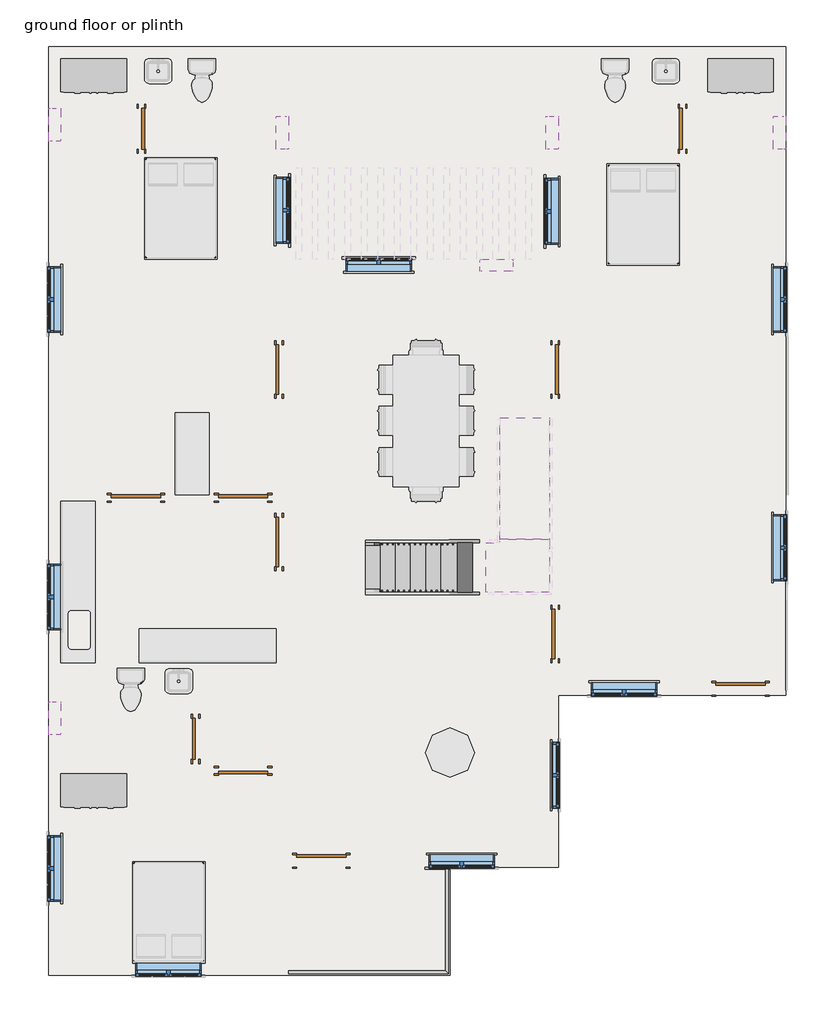
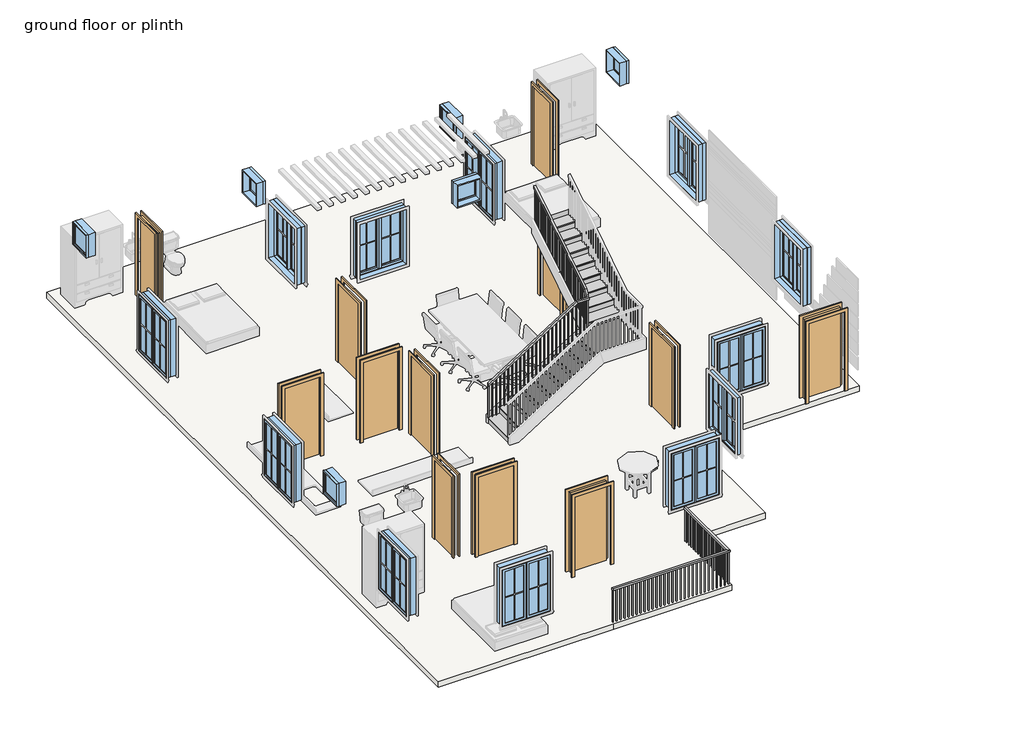
# One storey, part 1 of 3: 18 windows, 12 doors, 2 railings, 2 slabs, 2 stair flights.
"""IFC4 building model written with IfcOpenShell, lengths in millimetres."""

from ifc_helpers import new_model, si_unit, frame, origin, place, context, project, spatial, polyline, outline, extrude, faceted_brep, transform, mapped, element, save
from components import door_78caadf7, door_214872d5, door_e5f9f3c4, door_305aa2a5, door_0ca8825f, door_a90ba1ad, non_monolithic_landing_c5e4f846, stair_flight_fd6a9547, stair_flight_b3cbfaaf, window_80340324, window_8377141f, window_d9d3dda5

model = new_model("IFC4")

# Units and contexts
model_context = context("Model", 3, world=origin())
ifc_project = project(units=[si_unit("LENGTHUNIT", "METRE", prefix="MILLI")], contexts=[model_context])

# Site, building, storey
site = spatial("IfcSite", under=ifc_project)
building = spatial("IfcBuilding", under=site)
storey = spatial("IfcBuildingStorey", under=building, Name="ground floor or plinth", Elevation=609.6)

# Doors
placement = place(None, origin())
door_shape = door_78caadf7(model_context)
element("IfcDoor", 1, ObjectType="Single-Flush : 30\" x 84\"", at=placement, inside=storey, context=model_context, shape_type="MappedRepresentation", body=[
    mapped(door_shape, transform((3433.3423267, 4208.8496924, 609.6), x_axis=(0.0, -1.0, 0.0), y_axis=(1.0, 0.0, 0.0), z_axis=(0.0, 0.0, 1.0))),
])
element("IfcDoor", 2, ObjectType="Single-Flush : 30\" x 84\"", at=placement, inside=storey, context=model_context, shape_type="MappedRepresentation", body=[
    mapped(door_shape, transform((12463.0423267, 15511.8496924, 609.6), x_axis=(0.0, -1.0, 0.0), y_axis=(1.0, 0.0, 0.0), z_axis=(0.0, 0.0, 1.0))),
])
door_2_shape = door_214872d5(model_context)
element("IfcDoor", 3, ObjectType="Single-Flush : 30\" x 84\"", at=placement, inside=storey, context=model_context, shape_type="MappedRepresentation", body=[
    mapped(door_2_shape, transform((2430.0423267, 15511.8496924, 609.6), x_axis=(0.0, -1.0, 0.0), y_axis=(1.0, 0.0, 0.0), z_axis=(0.0, 0.0, 1.0))),
])
door_3_shape = door_e5f9f3c4(model_context)
element("IfcDoor", 4, ObjectType="Single-Flush : 36\" x 84\"", at=placement, inside=storey, context=model_context, shape_type="MappedRepresentation", body=[
    mapped(door_3_shape, transform((10100.8423267, 11054.1496924, 609.6), x_axis=(0.0, -1.0, 0.0), y_axis=(1.0, 0.0, 0.0), z_axis=(0.0, 0.0, 1.0))),
])
element("IfcDoor", 5, ObjectType="Single-Flush : 36\" x 84\"", at=placement, inside=storey, context=model_context, shape_type="MappedRepresentation", body=[
    mapped(door_3_shape, transform((2328.4423267, 8672.8996924, 609.6), x_axis=(1.0, 0.0, 0.0), y_axis=(0.0, 1.0, 0.0), z_axis=(0.0, 0.0, 1.0))),
])
element("IfcDoor", 6, ObjectType="Single-Flush : 36\" x 84\"", at=placement, inside=storey, context=model_context, shape_type="MappedRepresentation", body=[
    mapped(door_3_shape, transform((4315.9923267, 8672.8996924, 609.6), x_axis=(1.0, 0.0, 0.0), y_axis=(0.0, 1.0, 0.0), z_axis=(0.0, 0.0, 1.0))),
])
element("IfcDoor", 7, ObjectType="Single-Flush : 36\" x 84\"", at=placement, inside=storey, context=model_context, shape_type="MappedRepresentation", body=[
    mapped(door_3_shape, transform((10100.8423267, 6151.9496924, 609.6), x_axis=(0.0, 1.0, 0.0), y_axis=(-1.0, 0.0, 0.0), z_axis=(0.0, 0.0, 1.0))),
])
element("IfcDoor", 8, ObjectType="Single-Flush : 36\" x 84\"", at=placement, inside=storey, context=model_context, shape_type="MappedRepresentation", body=[
    mapped(door_3_shape, transform((4982.7423267, 7853.7496924, 609.6), x_axis=(0.0, 1.0, 0.0), y_axis=(-1.0, 0.0, 0.0), z_axis=(0.0, 0.0, 1.0))),
])
door_4_shape = door_305aa2a5(model_context)
element("IfcDoor", 9, ObjectType="Single-Flush : 36\" x 84\"", at=placement, inside=storey, context=model_context, shape_type="MappedRepresentation", body=[
    mapped(door_4_shape, transform((4982.7423267, 11054.1496924, 609.6), x_axis=(0.0, -1.0, 0.0), y_axis=(1.0, 0.0, 0.0), z_axis=(0.0, 0.0, 1.0))),
])
element("IfcDoor", 10, ObjectType="Single-Flush : 36\" x 84\"", at=placement, inside=storey, context=model_context, shape_type="MappedRepresentation", body=[
    mapped(door_4_shape, transform((4315.9923267, 3618.2996924, 609.6), x_axis=(1.0, 0.0, 0.0), y_axis=(0.0, 1.0, 0.0), z_axis=(0.0, 0.0, 1.0))),
])
door_5_shape = door_0ca8825f(model_context)
element("IfcDoor", 11, ObjectType="Single-Flush : 36\" x 84\"", at=placement, inside=storey, context=model_context, shape_type="MappedRepresentation", body=[
    mapped(door_5_shape, transform((13536.1923267, 5135.9496924, 609.6), x_axis=(1.0, 0.0, 0.0), y_axis=(0.0, 1.0, 0.0), z_axis=(0.0, 0.0, 1.0))),
])
door_6_shape = door_a90ba1ad(model_context)
element("IfcDoor", 12, ObjectType="Single-Flush : 36\" x 84\"", at=placement, inside=storey, context=model_context, shape_type="MappedRepresentation", body=[
    mapped(door_6_shape, transform((5763.7923267, 1948.2496924, 609.6), x_axis=(-1.0, 0.0, 0.0), y_axis=(0.0, -1.0, 0.0), z_axis=(0.0, 0.0, 1.0))),
])

# Railings
element("IfcRailing", 13, ObjectType="Handrail - Rectangular", at=placement, inside=storey, context=model_context, shape_type="SolidModel", body=[
    faceted_brep([(5154.1923267, -90.1003076, 1524.0), (5154.1923267, -90.1003076, 1473.2), (5154.1923267, -140.9003076, 1473.2), (5154.1923267, -140.9003076, 1524.0), (8068.8423267, -90.1003076, 1524.0), (8068.8423267, -90.1003076, 1473.2), (8119.6423267, -140.9003076, 1473.2), (8119.6423267, -140.9003076, 1524.0), (8068.8423267, 1795.8496924, 1524.0), (8119.6423267, 1795.8496924, 1524.0), (8119.6423267, 1795.8496924, 1473.2), (8068.8423267, 1795.8496924, 1473.2)], [[[0, 1, 2, 3]], [[1, 0, 4, 5]], [[2, 1, 5, 6]], [[3, 2, 6, 7]], [[0, 3, 7, 4]], [[8, 9, 10, 11]], [[5, 4, 8, 11]], [[6, 5, 11, 10]], [[7, 6, 10, 9]], [[4, 7, 9, 8]]]),
    extrude(outline(polyline([(8103.7673267, 1703.7746924), (8084.7173267, 1703.7746924), (8084.7173267, 1722.8246924), (8103.7673267, 1722.8246924), (8103.7673267, 1703.7746924)])), frame((0.0, 0.0, 609.6), z_axis=(0.0, 0.0, 1.0), x_axis=(1.0, 0.0, 0.0)), (0.0, 0.0, 1.0), 863.6),
    extrude(outline(polyline([(8103.7673267, 1602.1746924), (8084.7173267, 1602.1746924), (8084.7173267, 1621.2246924), (8103.7673267, 1621.2246924), (8103.7673267, 1602.1746924)])), frame((0.0, 0.0, 609.6), z_axis=(0.0, 0.0, 1.0), x_axis=(1.0, 0.0, 0.0)), (0.0, 0.0, 1.0), 863.6),
    extrude(outline(polyline([(8103.7673267, 1500.5746924), (8084.7173267, 1500.5746924), (8084.7173267, 1519.6246924), (8103.7673267, 1519.6246924), (8103.7673267, 1500.5746924)])), frame((0.0, 0.0, 609.6), z_axis=(0.0, 0.0, 1.0), x_axis=(1.0, 0.0, 0.0)), (0.0, 0.0, 1.0), 863.6),
    extrude(outline(polyline([(8103.7673267, 1398.9746924), (8084.7173267, 1398.9746924), (8084.7173267, 1418.0246924), (8103.7673267, 1418.0246924), (8103.7673267, 1398.9746924)])), frame((0.0, 0.0, 609.6), z_axis=(0.0, 0.0, 1.0), x_axis=(1.0, 0.0, 0.0)), (0.0, 0.0, 1.0), 863.6),
    extrude(outline(polyline([(8103.7673267, 1297.3746924), (8084.7173267, 1297.3746924), (8084.7173267, 1316.4246924), (8103.7673267, 1316.4246924), (8103.7673267, 1297.3746924)])), frame((0.0, 0.0, 609.6), z_axis=(0.0, 0.0, 1.0), x_axis=(1.0, 0.0, 0.0)), (0.0, 0.0, 1.0), 863.6),
    extrude(outline(polyline([(8103.7673267, 1195.7746924), (8084.7173267, 1195.7746924), (8084.7173267, 1214.8246924), (8103.7673267, 1214.8246924), (8103.7673267, 1195.7746924)])), frame((0.0, 0.0, 609.6), z_axis=(0.0, 0.0, 1.0), x_axis=(1.0, 0.0, 0.0)), (0.0, 0.0, 1.0), 863.6),
    extrude(outline(polyline([(8103.7673267, 1094.1746924), (8084.7173267, 1094.1746924), (8084.7173267, 1113.2246924), (8103.7673267, 1113.2246924), (8103.7673267, 1094.1746924)])), frame((0.0, 0.0, 609.6), z_axis=(0.0, 0.0, 1.0), x_axis=(1.0, 0.0, 0.0)), (0.0, 0.0, 1.0), 863.6),
    extrude(outline(polyline([(8103.7673267, 992.5746924), (8084.7173267, 992.5746924), (8084.7173267, 1011.6246924), (8103.7673267, 1011.6246924), (8103.7673267, 992.5746924)])), frame((0.0, 0.0, 609.6), z_axis=(0.0, 0.0, 1.0), x_axis=(1.0, 0.0, 0.0)), (0.0, 0.0, 1.0), 863.6),
    extrude(outline(polyline([(8103.7673267, 890.9746924), (8084.7173267, 890.9746924), (8084.7173267, 910.0246924), (8103.7673267, 910.0246924), (8103.7673267, 890.9746924)])), frame((0.0, 0.0, 609.6), z_axis=(0.0, 0.0, 1.0), x_axis=(1.0, 0.0, 0.0)), (0.0, 0.0, 1.0), 863.6),
    extrude(outline(polyline([(8103.7673267, 789.3746924), (8084.7173267, 789.3746924), (8084.7173267, 808.4246924), (8103.7673267, 808.4246924), (8103.7673267, 789.3746924)])), frame((0.0, 0.0, 609.6), z_axis=(0.0, 0.0, 1.0), x_axis=(1.0, 0.0, 0.0)), (0.0, 0.0, 1.0), 863.6),
    extrude(outline(polyline([(8103.7673267, 687.7746924), (8084.7173267, 687.7746924), (8084.7173267, 706.8246924), (8103.7673267, 706.8246924), (8103.7673267, 687.7746924)])), frame((0.0, 0.0, 609.6), z_axis=(0.0, 0.0, 1.0), x_axis=(1.0, 0.0, 0.0)), (0.0, 0.0, 1.0), 863.6),
    extrude(outline(polyline([(8103.7673267, 586.1746924), (8084.7173267, 586.1746924), (8084.7173267, 605.2246924), (8103.7673267, 605.2246924), (8103.7673267, 586.1746924)])), frame((0.0, 0.0, 609.6), z_axis=(0.0, 0.0, 1.0), x_axis=(1.0, 0.0, 0.0)), (0.0, 0.0, 1.0), 863.6),
    extrude(outline(polyline([(8103.7673267, 484.5746924), (8084.7173267, 484.5746924), (8084.7173267, 503.6246924), (8103.7673267, 503.6246924), (8103.7673267, 484.5746924)])), frame((0.0, 0.0, 609.6), z_axis=(0.0, 0.0, 1.0), x_axis=(1.0, 0.0, 0.0)), (0.0, 0.0, 1.0), 863.6),
    extrude(outline(polyline([(8103.7673267, 382.9746924), (8084.7173267, 382.9746924), (8084.7173267, 402.0246924), (8103.7673267, 402.0246924), (8103.7673267, 382.9746924)])), frame((0.0, 0.0, 609.6), z_axis=(0.0, 0.0, 1.0), x_axis=(1.0, 0.0, 0.0)), (0.0, 0.0, 1.0), 863.6),
    extrude(outline(polyline([(8103.7673267, 281.3746924), (8084.7173267, 281.3746924), (8084.7173267, 300.4246924), (8103.7673267, 300.4246924), (8103.7673267, 281.3746924)])), frame((0.0, 0.0, 609.6), z_axis=(0.0, 0.0, 1.0), x_axis=(1.0, 0.0, 0.0)), (0.0, 0.0, 1.0), 863.6),
    extrude(outline(polyline([(8103.7673267, 179.7746924), (8084.7173267, 179.7746924), (8084.7173267, 198.8246924), (8103.7673267, 198.8246924), (8103.7673267, 179.7746924)])), frame((0.0, 0.0, 609.6), z_axis=(0.0, 0.0, 1.0), x_axis=(1.0, 0.0, 0.0)), (0.0, 0.0, 1.0), 863.6),
    extrude(outline(polyline([(8103.7673267, 78.1746924), (8084.7173267, 78.1746924), (8084.7173267, 97.2246924), (8103.7673267, 97.2246924), (8103.7673267, 78.1746924)])), frame((0.0, 0.0, 609.6), z_axis=(0.0, 0.0, 1.0), x_axis=(1.0, 0.0, 0.0)), (0.0, 0.0, 1.0), 863.6),
    extrude(outline(polyline([(8103.7673267, -23.4253076), (8084.7173267, -23.4253076), (8084.7173267, -4.3753076), (8103.7673267, -4.3753076), (8103.7673267, -23.4253076)])), frame((0.0, 0.0, 609.6), z_axis=(0.0, 0.0, 1.0), x_axis=(1.0, 0.0, 0.0)), (0.0, 0.0, 1.0), 863.6),
    extrude(outline(polyline([(7989.4673267, -125.0253076), (7989.4673267, -105.9753076), (8008.5173267, -105.9753076), (8008.5173267, -125.0253076), (7989.4673267, -125.0253076)])), frame((0.0, 0.0, 609.6), z_axis=(0.0, 0.0, 1.0), x_axis=(1.0, 0.0, 0.0)), (0.0, 0.0, 1.0), 863.6),
    extrude(outline(polyline([(7887.8673267, -125.0253076), (7887.8673267, -105.9753076), (7906.9173267, -105.9753076), (7906.9173267, -125.0253076), (7887.8673267, -125.0253076)])), frame((0.0, 0.0, 609.6), z_axis=(0.0, 0.0, 1.0), x_axis=(1.0, 0.0, 0.0)), (0.0, 0.0, 1.0), 863.6),
    extrude(outline(polyline([(7786.2673267, -125.0253076), (7786.2673267, -105.9753076), (7805.3173267, -105.9753076), (7805.3173267, -125.0253076), (7786.2673267, -125.0253076)])), frame((0.0, 0.0, 609.6), z_axis=(0.0, 0.0, 1.0), x_axis=(1.0, 0.0, 0.0)), (0.0, 0.0, 1.0), 863.6),
    extrude(outline(polyline([(7684.6673267, -125.0253076), (7684.6673267, -105.9753076), (7703.7173267, -105.9753076), (7703.7173267, -125.0253076), (7684.6673267, -125.0253076)])), frame((0.0, 0.0, 609.6), z_axis=(0.0, 0.0, 1.0), x_axis=(1.0, 0.0, 0.0)), (0.0, 0.0, 1.0), 863.6),
    extrude(outline(polyline([(7583.0673267, -125.0253076), (7583.0673267, -105.9753076), (7602.1173267, -105.9753076), (7602.1173267, -125.0253076), (7583.0673267, -125.0253076)])), frame((0.0, 0.0, 609.6), z_axis=(0.0, 0.0, 1.0), x_axis=(1.0, 0.0, 0.0)), (0.0, 0.0, 1.0), 863.6),
    extrude(outline(polyline([(7481.4673267, -125.0253076), (7481.4673267, -105.9753076), (7500.5173267, -105.9753076), (7500.5173267, -125.0253076), (7481.4673267, -125.0253076)])), frame((0.0, 0.0, 609.6), z_axis=(0.0, 0.0, 1.0), x_axis=(1.0, 0.0, 0.0)), (0.0, 0.0, 1.0), 863.6),
    extrude(outline(polyline([(7379.8673267, -125.0253076), (7379.8673267, -105.9753076), (7398.9173267, -105.9753076), (7398.9173267, -125.0253076), (7379.8673267, -125.0253076)])), frame((0.0, 0.0, 609.6), z_axis=(0.0, 0.0, 1.0), x_axis=(1.0, 0.0, 0.0)), (0.0, 0.0, 1.0), 863.6),
    extrude(outline(polyline([(7278.2673267, -125.0253076), (7278.2673267, -105.9753076), (7297.3173267, -105.9753076), (7297.3173267, -125.0253076), (7278.2673267, -125.0253076)])), frame((0.0, 0.0, 609.6), z_axis=(0.0, 0.0, 1.0), x_axis=(1.0, 0.0, 0.0)), (0.0, 0.0, 1.0), 863.6),
    extrude(outline(polyline([(7176.6673267, -125.0253076), (7176.6673267, -105.9753076), (7195.7173267, -105.9753076), (7195.7173267, -125.0253076), (7176.6673267, -125.0253076)])), frame((0.0, 0.0, 609.6), z_axis=(0.0, 0.0, 1.0), x_axis=(1.0, 0.0, 0.0)), (0.0, 0.0, 1.0), 863.6),
    extrude(outline(polyline([(7075.0673267, -125.0253076), (7075.0673267, -105.9753076), (7094.1173267, -105.9753076), (7094.1173267, -125.0253076), (7075.0673267, -125.0253076)])), frame((0.0, 0.0, 609.6), z_axis=(0.0, 0.0, 1.0), x_axis=(1.0, 0.0, 0.0)), (0.0, 0.0, 1.0), 863.6),
    extrude(outline(polyline([(6973.4673267, -125.0253076), (6973.4673267, -105.9753076), (6992.5173267, -105.9753076), (6992.5173267, -125.0253076), (6973.4673267, -125.0253076)])), frame((0.0, 0.0, 609.6), z_axis=(0.0, 0.0, 1.0), x_axis=(1.0, 0.0, 0.0)), (0.0, 0.0, 1.0), 863.6),
    extrude(outline(polyline([(6871.8673267, -125.0253076), (6871.8673267, -105.9753076), (6890.9173267, -105.9753076), (6890.9173267, -125.0253076), (6871.8673267, -125.0253076)])), frame((0.0, 0.0, 609.6), z_axis=(0.0, 0.0, 1.0), x_axis=(1.0, 0.0, 0.0)), (0.0, 0.0, 1.0), 863.6),
    extrude(outline(polyline([(6770.2673267, -125.0253076), (6770.2673267, -105.9753076), (6789.3173267, -105.9753076), (6789.3173267, -125.0253076), (6770.2673267, -125.0253076)])), frame((0.0, 0.0, 609.6), z_axis=(0.0, 0.0, 1.0), x_axis=(1.0, 0.0, 0.0)), (0.0, 0.0, 1.0), 863.6),
    extrude(outline(polyline([(6668.6673267, -125.0253076), (6668.6673267, -105.9753076), (6687.7173267, -105.9753076), (6687.7173267, -125.0253076), (6668.6673267, -125.0253076)])), frame((0.0, 0.0, 609.6), z_axis=(0.0, 0.0, 1.0), x_axis=(1.0, 0.0, 0.0)), (0.0, 0.0, 1.0), 863.6),
    extrude(outline(polyline([(6567.0673267, -125.0253076), (6567.0673267, -105.9753076), (6586.1173267, -105.9753076), (6586.1173267, -125.0253076), (6567.0673267, -125.0253076)])), frame((0.0, 0.0, 609.6), z_axis=(0.0, 0.0, 1.0), x_axis=(1.0, 0.0, 0.0)), (0.0, 0.0, 1.0), 863.6),
    extrude(outline(polyline([(6465.4673267, -125.0253076), (6465.4673267, -105.9753076), (6484.5173267, -105.9753076), (6484.5173267, -125.0253076), (6465.4673267, -125.0253076)])), frame((0.0, 0.0, 609.6), z_axis=(0.0, 0.0, 1.0), x_axis=(1.0, 0.0, 0.0)), (0.0, 0.0, 1.0), 863.6),
    extrude(outline(polyline([(6363.8673267, -125.0253076), (6363.8673267, -105.9753076), (6382.9173267, -105.9753076), (6382.9173267, -125.0253076), (6363.8673267, -125.0253076)])), frame((0.0, 0.0, 609.6), z_axis=(0.0, 0.0, 1.0), x_axis=(1.0, 0.0, 0.0)), (0.0, 0.0, 1.0), 863.6),
    extrude(outline(polyline([(6262.2673267, -125.0253076), (6262.2673267, -105.9753076), (6281.3173267, -105.9753076), (6281.3173267, -125.0253076), (6262.2673267, -125.0253076)])), frame((0.0, 0.0, 609.6), z_axis=(0.0, 0.0, 1.0), x_axis=(1.0, 0.0, 0.0)), (0.0, 0.0, 1.0), 863.6),
    extrude(outline(polyline([(6160.6673267, -125.0253076), (6160.6673267, -105.9753076), (6179.7173267, -105.9753076), (6179.7173267, -125.0253076), (6160.6673267, -125.0253076)])), frame((0.0, 0.0, 609.6), z_axis=(0.0, 0.0, 1.0), x_axis=(1.0, 0.0, 0.0)), (0.0, 0.0, 1.0), 863.6),
    extrude(outline(polyline([(6059.0673267, -125.0253076), (6059.0673267, -105.9753076), (6078.1173267, -105.9753076), (6078.1173267, -125.0253076), (6059.0673267, -125.0253076)])), frame((0.0, 0.0, 609.6), z_axis=(0.0, 0.0, 1.0), x_axis=(1.0, 0.0, 0.0)), (0.0, 0.0, 1.0), 863.6),
    extrude(outline(polyline([(5957.4673267, -125.0253076), (5957.4673267, -105.9753076), (5976.5173267, -105.9753076), (5976.5173267, -125.0253076), (5957.4673267, -125.0253076)])), frame((0.0, 0.0, 609.6), z_axis=(0.0, 0.0, 1.0), x_axis=(1.0, 0.0, 0.0)), (0.0, 0.0, 1.0), 863.6),
    extrude(outline(polyline([(5855.8673267, -125.0253076), (5855.8673267, -105.9753076), (5874.9173267, -105.9753076), (5874.9173267, -125.0253076), (5855.8673267, -125.0253076)])), frame((0.0, 0.0, 609.6), z_axis=(0.0, 0.0, 1.0), x_axis=(1.0, 0.0, 0.0)), (0.0, 0.0, 1.0), 863.6),
    extrude(outline(polyline([(5754.2673267, -125.0253076), (5754.2673267, -105.9753076), (5773.3173267, -105.9753076), (5773.3173267, -125.0253076), (5754.2673267, -125.0253076)])), frame((0.0, 0.0, 609.6), z_axis=(0.0, 0.0, 1.0), x_axis=(1.0, 0.0, 0.0)), (0.0, 0.0, 1.0), 863.6),
    extrude(outline(polyline([(5652.6673267, -125.0253076), (5652.6673267, -105.9753076), (5671.7173267, -105.9753076), (5671.7173267, -125.0253076), (5652.6673267, -125.0253076)])), frame((0.0, 0.0, 609.6), z_axis=(0.0, 0.0, 1.0), x_axis=(1.0, 0.0, 0.0)), (0.0, 0.0, 1.0), 863.6),
    extrude(outline(polyline([(5551.0673267, -125.0253076), (5551.0673267, -105.9753076), (5570.1173267, -105.9753076), (5570.1173267, -125.0253076), (5551.0673267, -125.0253076)])), frame((0.0, 0.0, 609.6), z_axis=(0.0, 0.0, 1.0), x_axis=(1.0, 0.0, 0.0)), (0.0, 0.0, 1.0), 863.6),
    extrude(outline(polyline([(5449.4673267, -125.0253076), (5449.4673267, -105.9753076), (5468.5173267, -105.9753076), (5468.5173267, -125.0253076), (5449.4673267, -125.0253076)])), frame((0.0, 0.0, 609.6), z_axis=(0.0, 0.0, 1.0), x_axis=(1.0, 0.0, 0.0)), (0.0, 0.0, 1.0), 863.6),
    extrude(outline(polyline([(5347.8673267, -125.0253076), (5347.8673267, -105.9753076), (5366.9173267, -105.9753076), (5366.9173267, -125.0253076), (5347.8673267, -125.0253076)])), frame((0.0, 0.0, 609.6), z_axis=(0.0, 0.0, 1.0), x_axis=(1.0, 0.0, 0.0)), (0.0, 0.0, 1.0), 863.6),
    extrude(outline(polyline([(5246.2673267, -125.0253076), (5246.2673267, -105.9753076), (5265.3173267, -105.9753076), (5265.3173267, -125.0253076), (5246.2673267, -125.0253076)])), frame((0.0, 0.0, 609.6), z_axis=(0.0, 0.0, 1.0), x_axis=(1.0, 0.0, 0.0)), (0.0, 0.0, 1.0), 863.6),
    extrude(outline(polyline([(8084.7173267, -125.0253076), (8084.7173267, -105.9753076), (8103.7673267, -105.9753076), (8103.7673267, -125.0253076), (8084.7173267, -125.0253076)])), frame((0.0, 0.0, 609.6), z_axis=(0.0, 0.0, 1.0), x_axis=(1.0, 0.0, 0.0)), (0.0, 0.0, 1.0), 863.6),
    extrude(outline(polyline([(8103.7673267, 1776.7996924), (8084.7173267, 1776.7996924), (8084.7173267, 1795.8496924), (8103.7673267, 1795.8496924), (8103.7673267, 1776.7996924)])), frame((0.0, 0.0, 609.6), z_axis=(0.0, 0.0, 1.0), x_axis=(1.0, 0.0, 0.0)), (0.0, 0.0, 1.0), 863.6),
    extrude(outline(polyline([(5154.1923267, -125.0253076), (5154.1923267, -105.9753076), (5173.2423267, -105.9753076), (5173.2423267, -125.0253076), (5154.1923267, -125.0253076)])), frame((0.0, 0.0, 609.6), z_axis=(0.0, 0.0, 1.0), x_axis=(1.0, 0.0, 0.0)), (0.0, 0.0, 1.0), 863.6),
])
element("IfcRailing", 14, ObjectType="Handrail - Rectangular", at=placement, inside=storey, context=model_context, shape_type="SolidModel", body=[
    faceted_brep([(6584.2175025, 7843.0147181, 1701.8), (6584.2175025, 7843.0147181, 1641.586276), (6584.2175025, 7792.2147181, 1641.586276), (6584.2175025, 7792.2147181, 1701.8), (8819.4175025, 7843.0147181, 3124.2), (8834.2104975, 7843.0147181, 3073.4), (8834.2104975, 7792.2147181, 3073.4), (8819.4175025, 7792.2147181, 3124.2), (9129.2923267, 7843.0147181, 3124.2), (9129.2923267, 7792.2147181, 3124.2), (9129.2923267, 7792.2147181, 3073.4), (9129.2923267, 7843.0147181, 3073.4)], [[[0, 1, 2, 3]], [[1, 0, 4, 5]], [[2, 1, 5, 6]], [[3, 2, 6, 7]], [[0, 3, 7, 4]], [[8, 9, 10, 11]], [[5, 4, 8, 11]], [[6, 5, 11, 10]], [[7, 6, 10, 9]], [[4, 7, 9, 8]]]),
    faceted_brep([(9078.4923267, 7843.0147181, 3183.4666667), (9078.4923267, 7843.0147181, 3054.5062421), (9129.2923267, 7843.0147181, 3054.5062421), (9129.2923267, 7843.0147181, 3183.4666667), (9078.4923267, 7893.8147181, 3302.0), (9078.4923267, 7934.3261666, 3267.5662887), (9129.2923267, 7934.3261666, 3267.5662887), (9129.2923267, 7893.8147181, 3302.0), (9078.4923267, 10129.0147181, 4724.4), (9129.2923267, 10129.0147181, 4724.4), (9129.2923267, 10129.0147181, 4664.186276), (9078.4923267, 10129.0147181, 4664.186276)], [[[0, 1, 2, 3]], [[1, 0, 4, 5]], [[2, 1, 5, 6]], [[3, 2, 6, 7]], [[0, 3, 7, 4]], [[8, 9, 10, 11]], [[5, 4, 8, 11]], [[6, 5, 11, 10]], [[7, 6, 10, 9]], [[4, 7, 9, 8]]]),
    extrude(outline(polyline([(10036.9397181, 4605.5930941), (10036.9397181, 3632.2), (10017.8897181, 3632.2), (10017.8897181, 4593.4703669), (10036.9397181, 4605.5930941)])), frame((9094.3673267, 0.0, 0.0), z_axis=(1.0, 0.0, 0.0), x_axis=(0.0, 1.0, 0.0)), (0.0, 0.0, 1.0), 19.05),
    extrude(outline(polyline([(9935.3397181, 4540.9385487), (9935.3397181, 3632.2), (9916.2897181, 3632.2), (9916.2897181, 4528.8158214), (9935.3397181, 4540.9385487)])), frame((9094.3673267, 0.0, 0.0), z_axis=(1.0, 0.0, 0.0), x_axis=(0.0, 1.0, 0.0)), (0.0, 0.0, 1.0), 19.05),
    extrude(outline(polyline([(9833.7397181, 4476.2840032), (9833.7397181, 3454.4), (9814.6897181, 3454.4), (9814.6897181, 4464.161276), (9833.7397181, 4476.2840032)])), frame((9094.3673267, 0.0, 0.0), z_axis=(1.0, 0.0, 0.0), x_axis=(0.0, 1.0, 0.0)), (0.0, 0.0, 1.0), 19.05),
    extrude(outline(polyline([(9732.1397181, 4411.6294578), (9732.1397181, 3454.4), (9713.0897181, 3454.4), (9713.0897181, 4399.5067305), (9732.1397181, 4411.6294578)])), frame((9094.3673267, 0.0, 0.0), z_axis=(1.0, 0.0, 0.0), x_axis=(0.0, 1.0, 0.0)), (0.0, 0.0, 1.0), 19.05),
    extrude(outline(polyline([(9630.5397181, 4346.9749123), (9630.5397181, 3454.4), (9611.4897181, 3454.4), (9611.4897181, 4334.8521851), (9630.5397181, 4346.9749123)])), frame((9094.3673267, 0.0, 0.0), z_axis=(1.0, 0.0, 0.0), x_axis=(0.0, 1.0, 0.0)), (0.0, 0.0, 1.0), 19.05),
    extrude(outline(polyline([(9528.9397181, 4282.3203669), (9528.9397181, 3276.6), (9509.8897181, 3276.6), (9509.8897181, 4270.1976396), (9528.9397181, 4282.3203669)])), frame((9094.3673267, 0.0, 0.0), z_axis=(1.0, 0.0, 0.0), x_axis=(0.0, 1.0, 0.0)), (0.0, 0.0, 1.0), 19.05),
    extrude(outline(polyline([(9427.3397181, 4217.6658214), (9427.3397181, 3276.6), (9408.2897181, 3276.6), (9408.2897181, 4205.5430941), (9427.3397181, 4217.6658214)])), frame((9094.3673267, 0.0, 0.0), z_axis=(1.0, 0.0, 0.0), x_axis=(0.0, 1.0, 0.0)), (0.0, 0.0, 1.0), 19.05),
    extrude(outline(polyline([(9325.7397181, 4153.011276), (9325.7397181, 3276.6), (9306.6897181, 3276.6), (9306.6897181, 4140.8885487), (9325.7397181, 4153.011276)])), frame((9094.3673267, 0.0, 0.0), z_axis=(1.0, 0.0, 0.0), x_axis=(0.0, 1.0, 0.0)), (0.0, 0.0, 1.0), 19.05),
    extrude(outline(polyline([(9224.1397181, 4088.3567305), (9224.1397181, 3098.8), (9205.0897181, 3098.8), (9205.0897181, 4076.2340032), (9224.1397181, 4088.3567305)])), frame((9094.3673267, 0.0, 0.0), z_axis=(1.0, 0.0, 0.0), x_axis=(0.0, 1.0, 0.0)), (0.0, 0.0, 1.0), 19.05),
    extrude(outline(polyline([(9122.5397181, 4023.7021851), (9122.5397181, 3098.8), (9103.4897181, 3098.8), (9103.4897181, 4011.5794578), (9122.5397181, 4023.7021851)])), frame((9094.3673267, 0.0, 0.0), z_axis=(1.0, 0.0, 0.0), x_axis=(0.0, 1.0, 0.0)), (0.0, 0.0, 1.0), 19.05),
    extrude(outline(polyline([(9020.9397181, 3959.0476396), (9020.9397181, 3098.8), (9001.8897181, 3098.8), (9001.8897181, 3946.9249123), (9020.9397181, 3959.0476396)])), frame((9094.3673267, 0.0, 0.0), z_axis=(1.0, 0.0, 0.0), x_axis=(0.0, 1.0, 0.0)), (0.0, 0.0, 1.0), 19.05),
    extrude(outline(polyline([(8919.3397181, 3894.3930941), (8919.3397181, 2921.0), (8900.2897181, 2921.0), (8900.2897181, 3882.2703669), (8919.3397181, 3894.3930941)])), frame((9094.3673267, 0.0, 0.0), z_axis=(1.0, 0.0, 0.0), x_axis=(0.0, 1.0, 0.0)), (0.0, 0.0, 1.0), 19.05),
    extrude(outline(polyline([(8817.7397181, 3829.7385487), (8817.7397181, 2921.0), (8798.6897181, 2921.0), (8798.6897181, 3817.6158214), (8817.7397181, 3829.7385487)])), frame((9094.3673267, 0.0, 0.0), z_axis=(1.0, 0.0, 0.0), x_axis=(0.0, 1.0, 0.0)), (0.0, 0.0, 1.0), 19.05),
    extrude(outline(polyline([(8716.1397181, 3765.0840032), (8716.1397181, 2743.2), (8697.0897181, 2743.2), (8697.0897181, 3752.961276), (8716.1397181, 3765.0840032)])), frame((9094.3673267, 0.0, 0.0), z_axis=(1.0, 0.0, 0.0), x_axis=(0.0, 1.0, 0.0)), (0.0, 0.0, 1.0), 19.05),
    extrude(outline(polyline([(8614.5397181, 3700.4294578), (8614.5397181, 2743.2), (8595.4897181, 2743.2), (8595.4897181, 3688.3067305), (8614.5397181, 3700.4294578)])), frame((9094.3673267, 0.0, 0.0), z_axis=(1.0, 0.0, 0.0), x_axis=(0.0, 1.0, 0.0)), (0.0, 0.0, 1.0), 19.05),
    extrude(outline(polyline([(8512.9397181, 3635.7749123), (8512.9397181, 2743.2), (8493.8897181, 2743.2), (8493.8897181, 3623.6521851), (8512.9397181, 3635.7749123)])), frame((9094.3673267, 0.0, 0.0), z_axis=(1.0, 0.0, 0.0), x_axis=(0.0, 1.0, 0.0)), (0.0, 0.0, 1.0), 19.05),
    extrude(outline(polyline([(8411.3397181, 3571.1203669), (8411.3397181, 2565.4), (8392.2897181, 2565.4), (8392.2897181, 3558.9976396), (8411.3397181, 3571.1203669)])), frame((9094.3673267, 0.0, 0.0), z_axis=(1.0, 0.0, 0.0), x_axis=(0.0, 1.0, 0.0)), (0.0, 0.0, 1.0), 19.05),
    extrude(outline(polyline([(8309.7397181, 3506.4658214), (8309.7397181, 2565.4), (8290.6897181, 2565.4), (8290.6897181, 3494.3430941), (8309.7397181, 3506.4658214)])), frame((9094.3673267, 0.0, 0.0), z_axis=(1.0, 0.0, 0.0), x_axis=(0.0, 1.0, 0.0)), (0.0, 0.0, 1.0), 19.05),
    extrude(outline(polyline([(8208.1397181, 3441.811276), (8208.1397181, 2565.4), (8189.0897181, 2565.4), (8189.0897181, 3429.6885487), (8208.1397181, 3441.811276)])), frame((9094.3673267, 0.0, 0.0), z_axis=(1.0, 0.0, 0.0), x_axis=(0.0, 1.0, 0.0)), (0.0, 0.0, 1.0), 19.05),
    extrude(outline(polyline([(8106.5397181, 3377.1567305), (8106.5397181, 2387.6), (8087.4897181, 2387.6), (8087.4897181, 3365.0340032), (8106.5397181, 3377.1567305)])), frame((9094.3673267, 0.0, 0.0), z_axis=(1.0, 0.0, 0.0), x_axis=(0.0, 1.0, 0.0)), (0.0, 0.0, 1.0), 19.05),
    extrude(outline(polyline([(8004.9397181, 3312.5021851), (8004.9397181, 2387.6), (7985.8897181, 2387.6), (7985.8897181, 3300.3794578), (8004.9397181, 3312.5021851)])), frame((9094.3673267, 0.0, 0.0), z_axis=(1.0, 0.0, 0.0), x_axis=(0.0, 1.0, 0.0)), (0.0, 0.0, 1.0), 19.05),
    extrude(outline(polyline([(9013.0925025, 7827.1397181), (9032.1425025, 7827.1397181), (9032.1425025, 7808.0897181), (9013.0925025, 7808.0897181), (9013.0925025, 7827.1397181)])), frame((0.0, 0.0, 2209.8), z_axis=(0.0, 0.0, 1.0), x_axis=(1.0, 0.0, 0.0)), (0.0, 0.0, 1.0), 863.6),
    extrude(outline(polyline([(8911.4925025, 7827.1397181), (8930.5425025, 7827.1397181), (8930.5425025, 7808.0897181), (8911.4925025, 7808.0897181), (8911.4925025, 7827.1397181)])), frame((0.0, 0.0, 2209.8), z_axis=(0.0, 0.0, 1.0), x_axis=(1.0, 0.0, 0.0)), (0.0, 0.0, 1.0), 863.6),
    extrude(outline(polyline([(2993.2703669, 8708.2925025), (2032.0, 8708.2925025), (2032.0, 8727.3425025), (3005.3930941, 8727.3425025), (2993.2703669, 8708.2925025)])), frame((0.0, 7808.0897181, 0.0), z_axis=(0.0, 1.0, 0.0), x_axis=(0.0, 0.0, 1.0)), (0.0, 0.0, 1.0), 19.05),
    extrude(outline(polyline([(2928.6158214, 8606.6925025), (2032.0, 8606.6925025), (2032.0, 8625.7425025), (2940.7385487, 8625.7425025), (2928.6158214, 8606.6925025)])), frame((0.0, 7808.0897181, 0.0), z_axis=(0.0, 1.0, 0.0), x_axis=(0.0, 0.0, 1.0)), (0.0, 0.0, 1.0), 19.05),
    extrude(outline(polyline([(2863.961276, 8505.0925025), (1854.2, 8505.0925025), (1854.2, 8524.1425025), (2876.0840032, 8524.1425025), (2863.961276, 8505.0925025)])), frame((0.0, 7808.0897181, 0.0), z_axis=(0.0, 1.0, 0.0), x_axis=(0.0, 0.0, 1.0)), (0.0, 0.0, 1.0), 19.05),
    extrude(outline(polyline([(2799.3067305, 8403.4925025), (1854.2, 8403.4925025), (1854.2, 8422.5425025), (2811.4294578, 8422.5425025), (2799.3067305, 8403.4925025)])), frame((0.0, 7808.0897181, 0.0), z_axis=(0.0, 1.0, 0.0), x_axis=(0.0, 0.0, 1.0)), (0.0, 0.0, 1.0), 19.05),
    extrude(outline(polyline([(2734.6521851, 8301.8925025), (1854.2, 8301.8925025), (1854.2, 8320.9425025), (2746.7749123, 8320.9425025), (2734.6521851, 8301.8925025)])), frame((0.0, 7808.0897181, 0.0), z_axis=(0.0, 1.0, 0.0), x_axis=(0.0, 0.0, 1.0)), (0.0, 0.0, 1.0), 19.05),
    extrude(outline(polyline([(2669.9976396, 8200.2925025), (1676.4, 8200.2925025), (1676.4, 8219.3425025), (2682.1203669, 8219.3425025), (2669.9976396, 8200.2925025)])), frame((0.0, 7808.0897181, 0.0), z_axis=(0.0, 1.0, 0.0), x_axis=(0.0, 0.0, 1.0)), (0.0, 0.0, 1.0), 19.05),
    extrude(outline(polyline([(2605.3430941, 8098.6925025), (1676.4, 8098.6925025), (1676.4, 8117.7425025), (2617.4658214, 8117.7425025), (2605.3430941, 8098.6925025)])), frame((0.0, 7808.0897181, 0.0), z_axis=(0.0, 1.0, 0.0), x_axis=(0.0, 0.0, 1.0)), (0.0, 0.0, 1.0), 19.05),
    extrude(outline(polyline([(2540.6885487, 7997.0925025), (1676.4, 7997.0925025), (1676.4, 8016.1425025), (2552.811276, 8016.1425025), (2540.6885487, 7997.0925025)])), frame((0.0, 7808.0897181, 0.0), z_axis=(0.0, 1.0, 0.0), x_axis=(0.0, 0.0, 1.0)), (0.0, 0.0, 1.0), 19.05),
    extrude(outline(polyline([(2476.0340032, 7895.4925025), (1498.6, 7895.4925025), (1498.6, 7914.5425025), (2488.1567305, 7914.5425025), (2476.0340032, 7895.4925025)])), frame((0.0, 7808.0897181, 0.0), z_axis=(0.0, 1.0, 0.0), x_axis=(0.0, 0.0, 1.0)), (0.0, 0.0, 1.0), 19.05),
    extrude(outline(polyline([(2411.3794578, 7793.8925025), (1498.6, 7793.8925025), (1498.6, 7812.9425025), (2423.5021851, 7812.9425025), (2411.3794578, 7793.8925025)])), frame((0.0, 7808.0897181, 0.0), z_axis=(0.0, 1.0, 0.0), x_axis=(0.0, 0.0, 1.0)), (0.0, 0.0, 1.0), 19.05),
    extrude(outline(polyline([(2346.7249123, 7692.2925025), (1498.6, 7692.2925025), (1498.6, 7711.3425025), (2358.8476396, 7711.3425025), (2346.7249123, 7692.2925025)])), frame((0.0, 7808.0897181, 0.0), z_axis=(0.0, 1.0, 0.0), x_axis=(0.0, 0.0, 1.0)), (0.0, 0.0, 1.0), 19.05),
    extrude(outline(polyline([(2282.0703669, 7590.6925025), (1320.8, 7590.6925025), (1320.8, 7609.7425025), (2294.1930941, 7609.7425025), (2282.0703669, 7590.6925025)])), frame((0.0, 7808.0897181, 0.0), z_axis=(0.0, 1.0, 0.0), x_axis=(0.0, 0.0, 1.0)), (0.0, 0.0, 1.0), 19.05),
    extrude(outline(polyline([(2217.4158214, 7489.0925025), (1320.8, 7489.0925025), (1320.8, 7508.1425025), (2229.5385487, 7508.1425025), (2217.4158214, 7489.0925025)])), frame((0.0, 7808.0897181, 0.0), z_axis=(0.0, 1.0, 0.0), x_axis=(0.0, 0.0, 1.0)), (0.0, 0.0, 1.0), 19.05),
    extrude(outline(polyline([(2152.761276, 7387.4925025), (1143.0, 7387.4925025), (1143.0, 7406.5425025), (2164.8840032, 7406.5425025), (2152.761276, 7387.4925025)])), frame((0.0, 7808.0897181, 0.0), z_axis=(0.0, 1.0, 0.0), x_axis=(0.0, 0.0, 1.0)), (0.0, 0.0, 1.0), 19.05),
    extrude(outline(polyline([(2088.1067305, 7285.8925025), (1143.0, 7285.8925025), (1143.0, 7304.9425025), (2100.2294578, 7304.9425025), (2088.1067305, 7285.8925025)])), frame((0.0, 7808.0897181, 0.0), z_axis=(0.0, 1.0, 0.0), x_axis=(0.0, 0.0, 1.0)), (0.0, 0.0, 1.0), 19.05),
    extrude(outline(polyline([(2023.4521851, 7184.2925025), (1143.0, 7184.2925025), (1143.0, 7203.3425025), (2035.5749123, 7203.3425025), (2023.4521851, 7184.2925025)])), frame((0.0, 7808.0897181, 0.0), z_axis=(0.0, 1.0, 0.0), x_axis=(0.0, 0.0, 1.0)), (0.0, 0.0, 1.0), 19.05),
    extrude(outline(polyline([(1958.7976396, 7082.6925025), (965.2, 7082.6925025), (965.2, 7101.7425025), (1970.9203669, 7101.7425025), (1958.7976396, 7082.6925025)])), frame((0.0, 7808.0897181, 0.0), z_axis=(0.0, 1.0, 0.0), x_axis=(0.0, 0.0, 1.0)), (0.0, 0.0, 1.0), 19.05),
    extrude(outline(polyline([(1894.1430941, 6981.0925025), (965.2, 6981.0925025), (965.2, 7000.1425025), (1906.2658214, 7000.1425025), (1894.1430941, 6981.0925025)])), frame((0.0, 7808.0897181, 0.0), z_axis=(0.0, 1.0, 0.0), x_axis=(0.0, 0.0, 1.0)), (0.0, 0.0, 1.0), 19.05),
    extrude(outline(polyline([(1829.4885487, 6879.4925025), (965.2, 6879.4925025), (965.2, 6898.5425025), (1841.611276, 6898.5425025), (1829.4885487, 6879.4925025)])), frame((0.0, 7808.0897181, 0.0), z_axis=(0.0, 1.0, 0.0), x_axis=(0.0, 0.0, 1.0)), (0.0, 0.0, 1.0), 19.05),
    extrude(outline(polyline([(1764.8340032, 6777.8925025), (787.4, 6777.8925025), (787.4, 6796.9425025), (1776.9567305, 6796.9425025), (1764.8340032, 6777.8925025)])), frame((0.0, 7808.0897181, 0.0), z_axis=(0.0, 1.0, 0.0), x_axis=(0.0, 0.0, 1.0)), (0.0, 0.0, 1.0), 19.05),
    extrude(outline(polyline([(1700.1794578, 6676.2925025), (787.4, 6676.2925025), (787.4, 6695.3425025), (1712.3021851, 6695.3425025), (1700.1794578, 6676.2925025)])), frame((0.0, 7808.0897181, 0.0), z_axis=(0.0, 1.0, 0.0), x_axis=(0.0, 0.0, 1.0)), (0.0, 0.0, 1.0), 19.05),
    extrude(outline(polyline([(7903.3397181, 3195.2645754), (7903.3397181, 2209.8), (7884.2897181, 2209.8), (7884.2897181, 3150.8145754), (7903.3397181, 3195.2645754)])), frame((9094.3673267, 0.0, 0.0), z_axis=(1.0, 0.0, 0.0), x_axis=(0.0, 1.0, 0.0)), (0.0, 0.0, 1.0), 19.05),
    extrude(outline(polyline([(9094.3673267, 7827.1397181), (9113.4173267, 7827.1397181), (9113.4173267, 7808.0897181), (9094.3673267, 7808.0897181), (9094.3673267, 7827.1397181)])), frame((0.0, 0.0, 2209.8), z_axis=(0.0, 0.0, 1.0), x_axis=(1.0, 0.0, 0.0)), (0.0, 0.0, 1.0), 863.6),
    extrude(outline(polyline([(3057.9249123, 8809.8925025), (2209.8, 8809.8925025), (2209.8, 8828.9425025), (3070.0476396, 8828.9425025), (3057.9249123, 8809.8925025)])), frame((0.0, 7808.0897181, 0.0), z_axis=(0.0, 1.0, 0.0), x_axis=(0.0, 0.0, 1.0)), (0.0, 0.0, 1.0), 19.05),
    extrude(outline(polyline([(10129.0147181, 4664.186276), (10129.0147181, 3632.2), (10109.9647181, 3632.2), (10109.9647181, 4652.0635487), (10129.0147181, 4664.186276)])), frame((9094.3673267, 0.0, 0.0), z_axis=(1.0, 0.0, 0.0), x_axis=(0.0, 1.0, 0.0)), (0.0, 0.0, 1.0), 19.05),
    extrude(outline(polyline([(1641.586276, 6584.2175025), (787.4, 6584.2175025), (787.4, 6603.2675025), (1653.7090032, 6603.2675025), (1641.586276, 6584.2175025)])), frame((0.0, 7808.0897181, 0.0), z_axis=(0.0, 1.0, 0.0), x_axis=(0.0, 0.0, 1.0)), (0.0, 0.0, 1.0), 19.05),
])

# Slabs
element("IfcSlab", 15, at=placement, inside=storey, context=model_context, shape_type="SweptSolid", body=[
    extrude(outline(polyline([(14374.3923267, 17035.8496924), (14374.3923267, 5021.6496924), (10157.9923267, 5021.6496924), (10157.9923267, 1833.9496924), (8151.3923267, 1833.9496924), (8151.3923267, -172.6503076), (5154.1923267, -172.6503076), (709.1923267, -172.6503076), (709.1923267, 17035.8496924), (14374.3923267, 17035.8496924)])), frame((0.0, 0.0, 457.2), z_axis=(0.0, 0.0, 1.0), x_axis=(1.0, 0.0, 0.0)), (0.0, 0.0, 1.0), 152.4),
])
non_monolithic_landing_shape = non_monolithic_landing_c5e4f846(model_context)
element("IfcSlab", 16, ObjectType="Non-Monolithic Landing", at=placement, inside=storey, context=model_context, shape_type="MappedRepresentation", body=[
    mapped(non_monolithic_landing_shape, transform((0.0, 0.0, 0.0), x_axis=(1.0, 0.0, 0.0), y_axis=(0.0, 1.0, 0.0), z_axis=(0.0, 0.0, 1.0))),
])

# Stair flights
stair_flight_shape = stair_flight_fd6a9547(model_context)
element("IfcStairFlight", 17, ObjectType="2\" Tread 1\" Nosing 1/4\" Riser", at=placement, inside=storey, context=model_context, shape_type="MappedRepresentation", body=[
    mapped(stair_flight_shape, transform((0.0, 0.0, 0.0), x_axis=(1.0, 0.0, 0.0), y_axis=(0.0, 1.0, 0.0), z_axis=(0.0, 0.0, 1.0))),
])
stair_flight_2_shape = stair_flight_b3cbfaaf(model_context)
element("IfcStairFlight", 18, ObjectType="2\" Tread 1\" Nosing 1/4\" Riser", at=placement, inside=storey, context=model_context, shape_type="MappedRepresentation", body=[
    mapped(stair_flight_2_shape, transform((0.0, 0.0, 0.0), x_axis=(1.0, 0.0, 0.0), y_axis=(0.0, 1.0, 0.0), z_axis=(0.0, 0.0, 1.0))),
])

# Windows
window_shape = window_80340324(model_context)
element("IfcWindow", 19, ObjectType="Fixed : 24\" x 24\"", at=placement, inside=storey, context=model_context, shape_type="MappedRepresentation", body=[
    mapped(window_shape, transform((5039.8923267, 15397.5496924, 1676.4), x_axis=(0.0, -1.0, 0.0), y_axis=(1.0, 0.0, 0.0), z_axis=(0.0, 0.0, 1.0))),
])
element("IfcWindow", 20, ObjectType="Fixed : 24\" x 24\"", at=placement, inside=storey, context=model_context, shape_type="MappedRepresentation", body=[
    mapped(window_shape, transform((10043.6923267, 15473.7496924, 1676.4), x_axis=(0.0, 1.0, 0.0), y_axis=(-1.0, 0.0, 0.0), z_axis=(0.0, 0.0, 1.0))),
])
element("IfcWindow", 21, ObjectType="Fixed : 24\" x 24\"", at=placement, inside=storey, context=model_context, shape_type="MappedRepresentation", body=[
    mapped(window_shape, transform((9053.0923267, 12984.5496924, 1676.4), x_axis=(1.0, 0.0, 0.0), y_axis=(0.0, 1.0, 0.0), z_axis=(0.0, 0.0, 1.0))),
])
element("IfcWindow", 22, ObjectType="Fixed : 24\" x 24\"", at=placement, inside=storey, context=model_context, shape_type="MappedRepresentation", body=[
    mapped(window_shape, transform((823.4923267, 4627.9496924, 1676.4), x_axis=(0.0, 1.0, 0.0), y_axis=(-1.0, 0.0, 0.0), z_axis=(0.0, 0.0, 1.0))),
])
element("IfcWindow", 23, ObjectType="Fixed : 24\" x 24\"", at=placement, inside=storey, context=model_context, shape_type="MappedRepresentation", body=[
    mapped(window_shape, transform((823.4923267, 15626.1496924, 1676.4), x_axis=(0.0, 1.0, 0.0), y_axis=(-1.0, 0.0, 0.0), z_axis=(0.0, 0.0, 1.0))),
])
element("IfcWindow", 24, ObjectType="Fixed : 24\" x 24\"", at=placement, inside=storey, context=model_context, shape_type="MappedRepresentation", body=[
    mapped(window_shape, transform((14260.0923267, 15397.5496924, 1676.4), x_axis=(0.0, -1.0, 0.0), y_axis=(1.0, 0.0, 0.0), z_axis=(0.0, 0.0, 1.0))),
])
window_2_shape = window_8377141f(model_context)
element("IfcWindow", 25, ObjectType="Window-Casement-Double : 48\" x 60\"", at=placement, inside=storey, context=model_context, shape_type="MappedRepresentation", body=[
    mapped(window_2_shape, transform((2931.6923267, -58.3503076, 609.6), x_axis=(-1.0, 0.0, 0.0), y_axis=(0.0, -1.0, 0.0), z_axis=(0.0, 0.0, 1.0))),
])
element("IfcWindow", 26, ObjectType="Window-Casement-Double : 48\" x 60\"", at=placement, inside=storey, context=model_context, shape_type="MappedRepresentation", body=[
    mapped(window_2_shape, transform((823.4923267, 6837.7496924, 609.6), x_axis=(0.0, 1.0, 0.0), y_axis=(-1.0, 0.0, 0.0), z_axis=(0.0, 0.0, 1.0))),
])
element("IfcWindow", 27, ObjectType="Window-Casement-Double : 48\" x 60\"", at=placement, inside=storey, context=model_context, shape_type="MappedRepresentation", body=[
    mapped(window_2_shape, transform((823.4923267, 12349.5496924, 609.6), x_axis=(0.0, 1.0, 0.0), y_axis=(-1.0, 0.0, 0.0), z_axis=(0.0, 0.0, 1.0))),
])
element("IfcWindow", 28, ObjectType="Window-Casement-Double : 48\" x 60\"", at=placement, inside=storey, context=model_context, shape_type="MappedRepresentation", body=[
    mapped(window_2_shape, transform((5039.8923267, 14000.5496924, 609.6), x_axis=(0.0, -1.0, 0.0), y_axis=(1.0, 0.0, 0.0), z_axis=(0.0, 0.0, 1.0))),
])
element("IfcWindow", 29, ObjectType="Window-Casement-Double : 48\" x 60\"", at=placement, inside=storey, context=model_context, shape_type="MappedRepresentation", body=[
    mapped(window_2_shape, transform((10043.6923267, 13981.4996924, 609.6), x_axis=(0.0, 1.0, 0.0), y_axis=(-1.0, 0.0, 0.0), z_axis=(0.0, 0.0, 1.0))),
])
element("IfcWindow", 30, ObjectType="Window-Casement-Double : 48\" x 60\"", at=placement, inside=storey, context=model_context, shape_type="MappedRepresentation", body=[
    mapped(window_2_shape, transform((14260.0923267, 12349.5496924, 609.6), x_axis=(0.0, -1.0, 0.0), y_axis=(1.0, 0.0, 0.0), z_axis=(0.0, 0.0, 1.0))),
])
element("IfcWindow", 31, ObjectType="Window-Casement-Double : 48\" x 60\"", at=placement, inside=storey, context=model_context, shape_type="MappedRepresentation", body=[
    mapped(window_2_shape, transform((14260.0923267, 7752.1496924, 609.6), x_axis=(0.0, -1.0, 0.0), y_axis=(1.0, 0.0, 0.0), z_axis=(0.0, 0.0, 1.0))),
])
element("IfcWindow", 32, ObjectType="Window-Casement-Double : 48\" x 60\"", at=placement, inside=storey, context=model_context, shape_type="MappedRepresentation", body=[
    mapped(window_2_shape, transform((8367.2923267, 1948.2496924, 609.6), x_axis=(-1.0, 0.0, 0.0), y_axis=(0.0, -1.0, 0.0), z_axis=(0.0, 0.0, 1.0))),
])
element("IfcWindow", 33, ObjectType="Window-Casement-Double : 48\" x 60\"", at=placement, inside=storey, context=model_context, shape_type="MappedRepresentation", body=[
    mapped(window_2_shape, transform((6830.5923267, 12984.5496924, 609.6), x_axis=(1.0, 0.0, 0.0), y_axis=(0.0, 1.0, 0.0), z_axis=(0.0, 0.0, 1.0))),
])
element("IfcWindow", 34, ObjectType="Window-Casement-Double : 48\" x 60\"", at=placement, inside=storey, context=model_context, shape_type="MappedRepresentation", body=[
    mapped(window_2_shape, transform((823.4923267, 1808.5496924, 609.6), x_axis=(0.0, 1.0, 0.0), y_axis=(-1.0, 0.0, 0.0), z_axis=(0.0, 0.0, 1.0))),
])
element("IfcWindow", 35, ObjectType="Window-Casement-Double : 48\" x 60\"", at=placement, inside=storey, context=model_context, shape_type="MappedRepresentation", body=[
    mapped(window_2_shape, transform((11377.1923267, 5135.9496924, 609.6), x_axis=(-1.0, 0.0, 0.0), y_axis=(0.0, -1.0, 0.0), z_axis=(0.0, 0.0, 1.0))),
])
window_3_shape = window_d9d3dda5(model_context)
element("IfcWindow", 36, ObjectType="Window-Casement-Double : 48\" x 60\"", at=placement, inside=storey, context=model_context, shape_type="MappedRepresentation", body=[
    mapped(window_3_shape, transform((10100.8423267, 3535.7496924, 609.6), x_axis=(0.0, -1.0, 0.0), y_axis=(1.0, 0.0, 0.0), z_axis=(0.0, 0.0, 1.0))),
])

save(model, "model.ifc")

# Revit data of these elements
# Type "Single-Flush : 30\" x 84\""
#   Type Mark = "4"
#   Construction Type Id = "MDOOR"
#   Assembly Code = "C1020"
#   Analytic Construction = "Metal"
#   Thickness = 0' - 2"
#   Heat Transfer Coefficient (U) = 0.651978 BTU/(h·ft²·°F)
#   Height = 7' - 0"
#   Trim Projection Ext = 0' - 1"
#   Trim Projection Int = 0' - 1"
#   Trim Width = 0' - 3"
#   Width = 2' - 6"
#   Define Thermal Properties by = 1
#   Define Thermal Properties by = 1
#   Door Material = Door - Panel
#   Frame Material = Door - Frame
#   Visual Light Transmittance = 0
#   Solar Heat Gain Coefficient = 0
#   Function = (empty or 0)
#   Wall Closure = (empty or 0)
# Type "Single-Flush : 36\" x 84\""
#   Type Mark = "1"
#   Construction Type Id = "MDOOR"
#   Assembly Code = "C1020"
#   Analytic Construction = "Metal"
#   Thickness = 0' - 2"
#   Heat Transfer Coefficient (U) = 0.651978 BTU/(h·ft²·°F)
#   Height = 7' - 0"
#   Trim Projection Ext = 0' - 1"
#   Trim Projection Int = 0' - 1"
#   Trim Width = 0' - 3"
#   Width = 3' - 0"
#   Define Thermal Properties by = 1
#   Define Thermal Properties by = 1
#   Door Material = Door - Panel
#   Frame Material = Door - Frame
#   Visual Light Transmittance = 0
#   Solar Heat Gain Coefficient = 0
#   Function = (empty or 0)
#   Wall Closure = (empty or 0)
# Type "Handrail - Rectangular"
#   Assembly Code = "C2010400"
#   built-in parameter 1008612 = 0.0416667 (stored number, unit not read)
#   built-in parameter 1008611 = 0.0416667 (stored number, unit not read)
#   built-in parameter 1008609 = 0.333333 (stored number, unit not read)
#   built-in parameter 1008604 = 0.166667 (stored number, unit not read)
#   built-in parameter 1008603 = 0.166667 (stored number, unit not read)
#   Railing Height = 3' - 0"
#   built-in parameter 1008630 = 2
#   built-in parameter 1008610 = 2
#   built-in parameter 1008618 = Baluster - Square : 3/4"
# Type
#   Assembly Code = "B1010"
#   Function = 0
#   Layers, outside or top first: 0' - 6" "Concrete, Cast-in-Place gray" (function 1)
# Type "Fixed : 24\" x 24\""
#   Type Mark = "3"
#   Construction Type Id = "GSP4R"
#   Assembly Code = "B2020100"
#   Analytic Construction = "1/8 in Pilkington single glazing"
#   Visual Light Transmittance = 0.9
#   Solar Heat Gain Coefficient = 0.78
#   Heat Transfer Coefficient (U) = 0.6496 BTU/(h·ft²·°F)
#   Height = 2' - 0"
#   Default Sill Height = 3' - 0"
#   Width = 2' - 0"
#   Window Inset = 0' - 0 3/4"
#   Define Thermal Properties by = 1
#   Define Thermal Properties by = 1
#   Glass Pane Material = Glass
#   Sash Material = Sash
#   Wall Closure = (empty or 0)
# Type "Window-Casement-Double : 48\" x 60\""
#   Type Mark = "16"
#   Fire Rating = "0.5h"
#   Assembly Code = "B2020100"
#   Analytic Construction = "Double glazing - domestic"
#   Frame Extension [instance default] = 0' - 0 1/4"
#   Window Inset [instance default] = 0' - 0"
#   Wall Thickness [instance default] = 0' - 6"
#   Interior Wall Closure [instance default] = 0' - 2 1/4"
#   Half Width = 2' - 0"
#   Visual Light Transmittance = 0.81
#   Thermal Resistance (R) = 1.8146 (h·ft²·°F)/BTU
#   Solar Heat Gain Coefficient = 0.76
#   Rough Width = 4' - 0 1/2"
#   Rough Height = 5' - 0 1/2"
#   Height = 5' - 0"
#   Heat Transfer Coefficient (U) = 0.5511 BTU/(h·ft²·°F)
#   Exterior Wall Closure [instance default] = 0' - 1 1/4"
#   Extension Jamb [instance default] = 0' - 2 1/4"
#   Default Sill Height = 3' - 0"
#   Width = 4' - 0"
#   Define Thermal Properties by = 0
#   Muntin Visibility = yes
#   Interior Trim Visibility [instance default] = yes
#   Exterior Trim Visibility [instance default] = yes
#   Extension Jamb Visibility [instance default] = yes
#   Interior Trim Material = Wood - Stained
#   Muntin Pattern = Muntin Pattern_2x2 : Muntin Pattern_2x2
#   Interior Trim = Trim-Window-Interior-Flat : Picture Frame
#   Interior Frame Material = Wood - Stained
#   Glass Panel Material = Glass
#   Exterior Trim Material = Clad - White
#   Exterior Trim = Trim-Window-Exterior-Flat : with Sill
#   Exterior Frame Material = Clad - White
#   Wall Closure = (empty or 0)
# Elements 1, 2, 3 (IfcDoor, "Single-Flush : 30\" x 84\"")
#   Phase Created = New Construction
#   Materials on its faces: "Door - Frame", "Door - Panel"
# Elements 4, 5, 6, 7, 8, 9, 10, 11, 12 (IfcDoor, "Single-Flush : 36\" x 84\"")
#   Phase Created = New Construction
#   Materials on its faces: "Door - Frame", "Door - Panel"
# Elements 13, 14 (IfcRailing, "Handrail - Rectangular")
#   Phase Created = New Construction
# Element 15 (IfcSlab)
#   Height Offset From Level = 0' - 0"
#   Phase Created = New Construction
#   Materials on its faces: "Concrete, Cast-in-Place gray"
# Element 16 (IfcSlab, "Non-Monolithic Landing")
#   Phase Created = New Construction
# Elements 17, 18 (IfcStairFlight, "2\" Tread 1\" Nosing 1/4\" Riser")
#   Phase Created = New Construction
# Element 19 (IfcWindow, "Fixed : 24\" x 24\"")
#   Mark = "11"
#   Phase Created = New Construction
#   Materials on its faces: "Sash", "Glass"
# Element 20 (IfcWindow, "Fixed : 24\" x 24\"")
#   Mark = "12"
#   Phase Created = New Construction
#   Materials on its faces: "Sash", "Glass"
# Element 21 (IfcWindow, "Fixed : 24\" x 24\"")
#   Mark = "13"
#   Phase Created = New Construction
#   Materials on its faces: "Sash", "Glass"
# Element 22 (IfcWindow, "Fixed : 24\" x 24\"")
#   Mark = "14"
#   Phase Created = New Construction
#   Materials on its faces: "Sash", "Glass"
# Element 23 (IfcWindow, "Fixed : 24\" x 24\"")
#   Mark = "16"
#   Phase Created = New Construction
#   Materials on its faces: "Sash", "Glass"
# Element 24 (IfcWindow, "Fixed : 24\" x 24\"")
#   Mark = "17"
#   Phase Created = New Construction
#   Materials on its faces: "Sash", "Glass"
# Element 25 (IfcWindow, "Window-Casement-Double : 48\" x 60\"")
#   Mark = "1"
#   Window Inset = 0' - 0"
#   Interior Wall Closure = 0' - 2 1/4"
#   Frame Extension = 0' - 0 1/4"
#   Exterior Wall Closure = 0' - 1 1/4"
#   Interior Trim Visibility = yes
#   Exterior Trim Visibility = yes
#   Phase Created = New Construction
#   Materials on its faces: "Wood - Stained", "Glass", "Clad - White"
# Element 26 (IfcWindow, "Window-Casement-Double : 48\" x 60\"")
#   Mark = "2"
#   Window Inset = 0' - 0"
#   Interior Wall Closure = 0' - 2 1/4"
#   Frame Extension = 0' - 0 1/4"
#   Exterior Wall Closure = 0' - 1 1/4"
#   Interior Trim Visibility = yes
#   Exterior Trim Visibility = yes
#   Phase Created = New Construction
#   Materials on its faces: "Wood - Stained", "Glass", "Clad - White"
# Element 27 (IfcWindow, "Window-Casement-Double : 48\" x 60\"")
#   Mark = "3"
#   Window Inset = 0' - 0"
#   Interior Wall Closure = 0' - 2 1/4"
#   Frame Extension = 0' - 0 1/4"
#   Exterior Wall Closure = 0' - 1 1/4"
#   Interior Trim Visibility = yes
#   Exterior Trim Visibility = yes
#   Phase Created = New Construction
#   Materials on its faces: "Wood - Stained", "Glass", "Clad - White"
# Element 28 (IfcWindow, "Window-Casement-Double : 48\" x 60\"")
#   Mark = "4"
#   Window Inset = 0' - 0"
#   Interior Wall Closure = 0' - 2 1/4"
#   Frame Extension = 0' - 0 1/4"
#   Exterior Wall Closure = 0' - 1 1/4"
#   Interior Trim Visibility = yes
#   Exterior Trim Visibility = yes
#   Phase Created = New Construction
#   Materials on its faces: "Wood - Stained", "Glass", "Clad - White"
# Element 29 (IfcWindow, "Window-Casement-Double : 48\" x 60\"")
#   Mark = "5"
#   Window Inset = 0' - 0"
#   Interior Wall Closure = 0' - 2 1/4"
#   Frame Extension = 0' - 0 1/4"
#   Exterior Wall Closure = 0' - 1 1/4"
#   Interior Trim Visibility = yes
#   Exterior Trim Visibility = yes
#   Phase Created = New Construction
#   Materials on its faces: "Wood - Stained", "Glass", "Clad - White"
# Element 30 (IfcWindow, "Window-Casement-Double : 48\" x 60\"")
#   Mark = "6"
#   Window Inset = 0' - 0"
#   Interior Wall Closure = 0' - 2 1/4"
#   Frame Extension = 0' - 0 1/4"
#   Exterior Wall Closure = 0' - 1 1/4"
#   Interior Trim Visibility = yes
#   Exterior Trim Visibility = yes
#   Phase Created = New Construction
#   Materials on its faces: "Wood - Stained", "Glass", "Clad - White"
# Element 31 (IfcWindow, "Window-Casement-Double : 48\" x 60\"")
#   Mark = "7"
#   Window Inset = 0' - 0"
#   Interior Wall Closure = 0' - 2 1/4"
#   Frame Extension = 0' - 0 1/4"
#   Exterior Wall Closure = 0' - 1 1/4"
#   Interior Trim Visibility = yes
#   Exterior Trim Visibility = yes
#   Phase Created = New Construction
#   Materials on its faces: "Wood - Stained", "Glass", "Clad - White"
# Element 32 (IfcWindow, "Window-Casement-Double : 48\" x 60\"")
#   Mark = "8"
#   Window Inset = 0' - 0"
#   Interior Wall Closure = 0' - 2 1/4"
#   Frame Extension = 0' - 0 1/4"
#   Exterior Wall Closure = 0' - 1 1/4"
#   Interior Trim Visibility = yes
#   Exterior Trim Visibility = yes
#   Phase Created = New Construction
#   Materials on its faces: "Wood - Stained", "Glass", "Clad - White"
# Element 33 (IfcWindow, "Window-Casement-Double : 48\" x 60\"")
#   Mark = "10"
#   Window Inset = 0' - 0"
#   Interior Wall Closure = 0' - 2 1/4"
#   Frame Extension = 0' - 0 1/4"
#   Exterior Wall Closure = 0' - 1 1/4"
#   Interior Trim Visibility = yes
#   Exterior Trim Visibility = yes
#   Phase Created = New Construction
#   Materials on its faces: "Wood - Stained", "Glass", "Clad - White"
# Element 34 (IfcWindow, "Window-Casement-Double : 48\" x 60\"")
#   Mark = "15"
